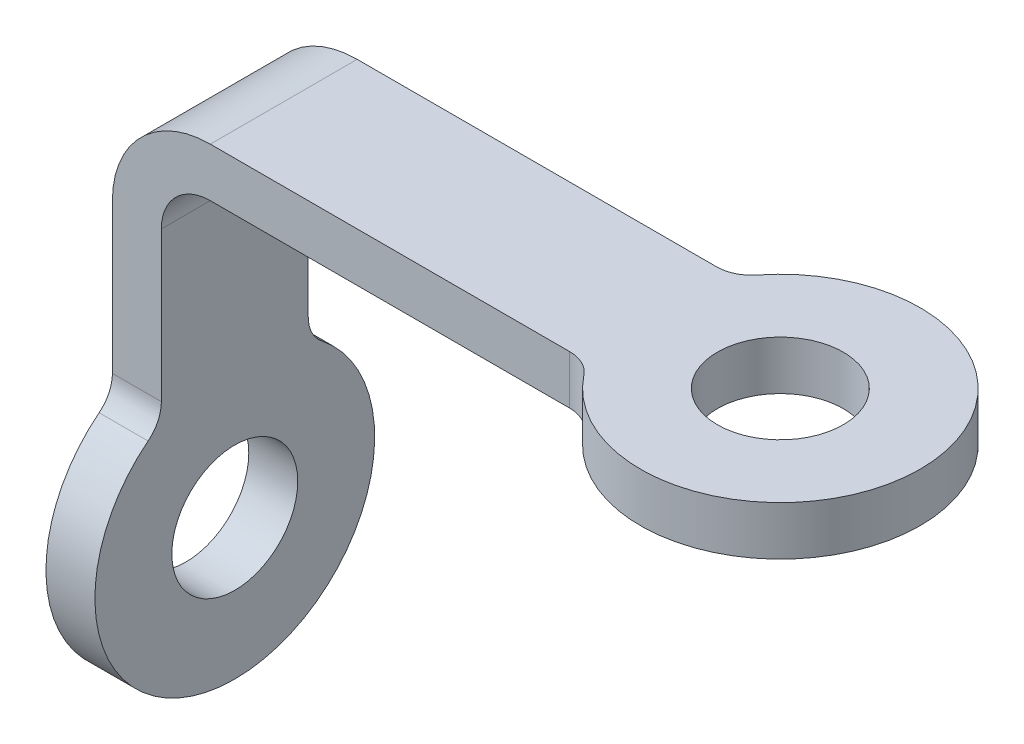
ISO-10303-21;
HEADER;
FILE_DESCRIPTION(('STEP AP214'),'2;1');
FILE_NAME('part.step','',(''),(''),'','','');
FILE_SCHEMA(('AUTOMOTIVE_DESIGN { 1 0 10303 214 1 1 1 1 }'));
ENDSEC;
DATA;
#1=APPLICATION_CONTEXT('core data for automotive mechanical design processes');
#2=APPLICATION_PROTOCOL_DEFINITION('international standard','automotive_design',2000,#1);
#3=PRODUCT_CONTEXT('',#1,'mechanical');
#4=PRODUCT('Part','Part','',(#3));
#5=PRODUCT_RELATED_PRODUCT_CATEGORY('part','',(#4));
#6=PRODUCT_DEFINITION_FORMATION('','',#4);
#7=PRODUCT_DEFINITION_CONTEXT('part definition',#1,'design');
#8=PRODUCT_DEFINITION('design','',#6,#7);
#9=PRODUCT_DEFINITION_SHAPE('','',#8);
#10=(LENGTH_UNIT() NAMED_UNIT(*) SI_UNIT(.MILLI.,.METRE.));
#11=(NAMED_UNIT(*) PLANE_ANGLE_UNIT() SI_UNIT($,.RADIAN.));
#12=(NAMED_UNIT(*) SI_UNIT($,.STERADIAN.) SOLID_ANGLE_UNIT());
#13=UNCERTAINTY_MEASURE_WITH_UNIT(LENGTH_MEASURE(1.E-05),#10,'distance_accuracy_value','');
#14=(GEOMETRIC_REPRESENTATION_CONTEXT(3) GLOBAL_UNCERTAINTY_ASSIGNED_CONTEXT((#13)) GLOBAL_UNIT_ASSIGNED_CONTEXT((#10,
#11,#12)) REPRESENTATION_CONTEXT('',''));
#15=CARTESIAN_POINT('',(0.,0.,0.));
#16=DIRECTION('',(0.,0.,1.));
#17=DIRECTION('',(1.,0.,0.));
#18=AXIS2_PLACEMENT_3D('',#15,#16,#17);
#19=CARTESIAN_POINT('',(0.,-7.,0.));
#20=DIRECTION('',(0.,1.,0.));
#21=DIRECTION('',(0.,0.,1.));
#22=AXIS2_PLACEMENT_3D('',#19,#20,#21);
#23=CYLINDRICAL_SURFACE('',#22,20.);
#24=CARTESIAN_POINT('',(0.,-7.,0.));
#25=DIRECTION('',(0.,1.,0.));
#26=DIRECTION('',(0.,0.,1.));
#27=AXIS2_PLACEMENT_3D('',#24,#25,#26);
#28=CIRCLE('',#27,20.);
#29=CARTESIAN_POINT('',(-15.6920361967464,-7.,12.4));
#30=VERTEX_POINT('',#29);
#31=CARTESIAN_POINT('',(-15.6920361967464,-7.,-12.4));
#32=VERTEX_POINT('',#31);
#33=EDGE_CURVE('E216',#30,#32,#28,.T.);
#34=ORIENTED_EDGE('',*,*,#33,.T.);
#35=DIRECTION('',(0.,1.,0.));
#36=VECTOR('',#35,1.);
#37=CARTESIAN_POINT('',(-15.6920361967464,-7.,-12.4));
#38=LINE('',#37,#36);
#39=CARTESIAN_POINT('',(-15.6920361967464,0.,-12.4));
#40=VERTEX_POINT('',#39);
#41=EDGE_CURVE('E149',#32,#40,#38,.T.);
#42=ORIENTED_EDGE('',*,*,#41,.T.);
#43=CARTESIAN_POINT('',(0.,0.,0.));
#44=DIRECTION('',(0.,1.,0.));
#45=DIRECTION('',(0.,0.,1.));
#46=AXIS2_PLACEMENT_3D('',#43,#44,#45);
#47=CIRCLE('',#46,20.);
#48=CARTESIAN_POINT('',(-15.6920361967464,0.,12.4));
#49=VERTEX_POINT('',#48);
#50=EDGE_CURVE('E135',#49,#40,#47,.T.);
#51=ORIENTED_EDGE('',*,*,#50,.F.);
#52=DIRECTION('',(0.,1.,0.));
#53=VECTOR('',#52,1.);
#54=CARTESIAN_POINT('',(-15.6920361967464,-7.,12.4));
#55=LINE('',#54,#53);
#56=EDGE_CURVE('E148',#49,#30,#55,.F.);
#57=ORIENTED_EDGE('',*,*,#56,.T.);
#58=EDGE_LOOP('',(#34,#42,#51,#57));
#59=FACE_BOUND('',#58,.T.);
#60=ADVANCED_FACE('F39',(#59),#23,.T.);
#61=CARTESIAN_POINT('',(-17.0220445305492,-7.,10.5));
#62=DIRECTION('',(0.,0.,1.));
#63=DIRECTION('',(1.,0.,0.));
#64=AXIS2_PLACEMENT_3D('',#61,#62,#63);
#65=PLANE('',#64);
#66=DIRECTION('',(1.,0.,0.));
#67=VECTOR('',#66,1.);
#68=CARTESIAN_POINT('',(-17.0220445305492,0.,10.5));
#69=LINE('',#68,#67);
#70=CARTESIAN_POINT('',(-71.,0.,10.5));
#71=VERTEX_POINT('',#70);
#72=CARTESIAN_POINT('',(-19.615045245933,0.,10.5));
#73=VERTEX_POINT('',#72);
#74=EDGE_CURVE('E134',#71,#73,#69,.T.);
#75=ORIENTED_EDGE('',*,*,#74,.F.);
#76=CARTESIAN_POINT('',(-71.,-14.,10.5));
#77=DIRECTION('',(0.,0.,1.));
#78=DIRECTION('',(1.,0.,0.));
#79=AXIS2_PLACEMENT_3D('',#76,#77,#78);
#80=CIRCLE('',#79,14.);
#81=CARTESIAN_POINT('',(-85.,-14.,10.5));
#82=VERTEX_POINT('',#81);
#83=EDGE_CURVE('E192',#71,#82,#80,.T.);
#84=ORIENTED_EDGE('',*,*,#83,.T.);
#85=DIRECTION('',(0.,1.,0.));
#86=VECTOR('',#85,1.);
#87=CARTESIAN_POINT('',(-85.,-7.,10.5));
#88=LINE('',#87,#86);
#89=CARTESIAN_POINT('',(-85.,-35.384954754067,10.5));
#90=VERTEX_POINT('',#89);
#91=EDGE_CURVE('E156',#90,#82,#88,.T.);
#92=ORIENTED_EDGE('',*,*,#91,.F.);
#93=DIRECTION('',(-1.,0.,0.));
#94=VECTOR('',#93,1.);
#95=CARTESIAN_POINT('',(-17.0220445305492,-35.384954754067,10.5));
#96=LINE('',#95,#94);
#97=CARTESIAN_POINT('',(-78.,-35.384954754067,10.4999999999999));
#98=VERTEX_POINT('',#97);
#99=EDGE_CURVE('E172',#90,#98,#96,.F.);
#100=ORIENTED_EDGE('',*,*,#99,.T.);
#101=DIRECTION('',(0.,-1.,0.));
#102=VECTOR('',#101,1.);
#103=CARTESIAN_POINT('',(-78.,0.,10.5));
#104=LINE('',#103,#102);
#105=CARTESIAN_POINT('',(-78.,-14.,10.5));
#106=VERTEX_POINT('',#105);
#107=EDGE_CURVE('E252',#106,#98,#104,.T.);
#108=ORIENTED_EDGE('',*,*,#107,.F.);
#109=CARTESIAN_POINT('',(-71.,-14.,10.5));
#110=DIRECTION('',(0.,0.,1.));
#111=DIRECTION('',(1.,0.,0.));
#112=AXIS2_PLACEMENT_3D('',#109,#110,#111);
#113=CIRCLE('',#112,7.);
#114=CARTESIAN_POINT('',(-71.,-7.,10.5));
#115=VERTEX_POINT('',#114);
#116=EDGE_CURVE('E11',#106,#115,#113,.F.);
#117=ORIENTED_EDGE('',*,*,#116,.T.);
#118=DIRECTION('',(1.,0.,0.));
#119=VECTOR('',#118,1.);
#120=CARTESIAN_POINT('',(-17.0220445305492,-7.,10.5));
#121=LINE('',#120,#119);
#122=CARTESIAN_POINT('',(-19.615045245933,-7.,10.5));
#123=VERTEX_POINT('',#122);
#124=EDGE_CURVE('E207',#115,#123,#121,.T.);
#125=ORIENTED_EDGE('',*,*,#124,.T.);
#126=DIRECTION('',(0.,-1.,0.));
#127=VECTOR('',#126,1.);
#128=CARTESIAN_POINT('',(-19.615045245933,0.,10.5));
#129=LINE('',#128,#127);
#130=EDGE_CURVE('E179',#123,#73,#129,.F.);
#131=ORIENTED_EDGE('',*,*,#130,.T.);
#132=EDGE_LOOP('',(#75,#84,#92,#100,#108,#117,#125,#131));
#133=FACE_BOUND('',#132,.T.);
#134=ADVANCED_FACE('F229',(#133),#65,.T.);
#135=CARTESIAN_POINT('',(-85.,-7.,-10.5));
#136=DIRECTION('',(-1.,0.,0.));
#137=DIRECTION('',(0.,0.,1.));
#138=AXIS2_PLACEMENT_3D('',#135,#136,#137);
#139=PLANE('',#138);
#140=ORIENTED_EDGE('',*,*,#91,.T.);
#141=DIRECTION('',(0.,0.,1.));
#142=VECTOR('',#141,1.);
#143=CARTESIAN_POINT('',(-85.,-14.,-10.5));
#144=LINE('',#143,#142);
#145=CARTESIAN_POINT('',(-85.,-14.,-10.5));
#146=VERTEX_POINT('',#145);
#147=EDGE_CURVE('E191',#82,#146,#144,.F.);
#148=ORIENTED_EDGE('',*,*,#147,.T.);
#149=DIRECTION('',(0.,1.,0.));
#150=VECTOR('',#149,1.);
#151=CARTESIAN_POINT('',(-85.,-7.,-10.5));
#152=LINE('',#151,#150);
#153=CARTESIAN_POINT('',(-85.,-35.3849547540669,-10.5));
#154=VERTEX_POINT('',#153);
#155=EDGE_CURVE('E161',#154,#146,#152,.T.);
#156=ORIENTED_EDGE('',*,*,#155,.F.);
#157=CARTESIAN_POINT('',(-85.,-35.3849547540669,-15.5));
#158=DIRECTION('',(-1.,0.,0.));
#159=DIRECTION('',(0.,0.,1.));
#160=AXIS2_PLACEMENT_3D('',#157,#158,#159);
#161=CIRCLE('',#160,5.);
#162=CARTESIAN_POINT('',(-85.,-39.3079638032535,-12.4));
#163=VERTEX_POINT('',#162);
#164=EDGE_CURVE('E181',#154,#163,#161,.F.);
#165=ORIENTED_EDGE('',*,*,#164,.T.);
#166=CARTESIAN_POINT('',(-85.,-55.,0.));
#167=DIRECTION('',(1.,0.,0.));
#168=DIRECTION('',(0.,0.,-1.));
#169=AXIS2_PLACEMENT_3D('',#166,#167,#168);
#170=CIRCLE('',#169,20.);
#171=CARTESIAN_POINT('',(-85.,-39.3079638032536,12.4));
#172=VERTEX_POINT('',#171);
#173=EDGE_CURVE('E236',#172,#163,#170,.T.);
#174=ORIENTED_EDGE('',*,*,#173,.F.);
#175=CARTESIAN_POINT('',(-85.,-35.384954754067,15.5));
#176=DIRECTION('',(-1.,0.,0.));
#177=DIRECTION('',(0.,0.,1.));
#178=AXIS2_PLACEMENT_3D('',#175,#176,#177);
#179=CIRCLE('',#178,5.);
#180=EDGE_CURVE('E190',#172,#90,#179,.F.);
#181=ORIENTED_EDGE('',*,*,#180,.T.);
#182=EDGE_LOOP('',(#140,#148,#156,#165,#174,#181));
#183=FACE_BOUND('',#182,.T.);
#184=CARTESIAN_POINT('',(-85.,-55.,0.));
#185=DIRECTION('',(1.,0.,0.));
#186=DIRECTION('',(0.,0.,-1.));
#187=AXIS2_PLACEMENT_3D('',#184,#185,#186);
#188=CIRCLE('',#187,9.);
#189=CARTESIAN_POINT('',(-85.,-55.,-9.00000000000006));
#190=VERTEX_POINT('',#189);
#191=EDGE_CURVE('E260',#190,#190,#188,.T.);
#192=ORIENTED_EDGE('',*,*,#191,.T.);
#193=EDGE_LOOP('',(#192));
#194=FACE_BOUND('',#193,.T.);
#195=ADVANCED_FACE('F232',(#183,#194),#139,.T.);
#196=CARTESIAN_POINT('',(-17.0220445305492,-7.,-10.5));
#197=DIRECTION('',(0.,0.,-1.));
#198=DIRECTION('',(-1.,0.,0.));
#199=AXIS2_PLACEMENT_3D('',#196,#197,#198);
#200=PLANE('',#199);
#201=ORIENTED_EDGE('',*,*,#155,.T.);
#202=CARTESIAN_POINT('',(-71.,-14.,-10.5));
#203=DIRECTION('',(0.,0.,-1.));
#204=DIRECTION('',(-1.,0.,0.));
#205=AXIS2_PLACEMENT_3D('',#202,#203,#204);
#206=CIRCLE('',#205,14.);
#207=CARTESIAN_POINT('',(-71.,0.,-10.5));
#208=VERTEX_POINT('',#207);
#209=EDGE_CURVE('E197',#146,#208,#206,.T.);
#210=ORIENTED_EDGE('',*,*,#209,.T.);
#211=DIRECTION('',(-1.,0.,0.));
#212=VECTOR('',#211,1.);
#213=CARTESIAN_POINT('',(-17.0220445305492,0.,-10.5));
#214=LINE('',#213,#212);
#215=CARTESIAN_POINT('',(-19.615045245933,0.,-10.5));
#216=VERTEX_POINT('',#215);
#217=EDGE_CURVE('E147',#216,#208,#214,.T.);
#218=ORIENTED_EDGE('',*,*,#217,.F.);
#219=DIRECTION('',(0.,-1.,0.));
#220=VECTOR('',#219,1.);
#221=CARTESIAN_POINT('',(-19.615045245933,-7.,-10.5));
#222=LINE('',#221,#220);
#223=CARTESIAN_POINT('',(-19.615045245933,-7.,-10.5));
#224=VERTEX_POINT('',#223);
#225=EDGE_CURVE('E170',#216,#224,#222,.T.);
#226=ORIENTED_EDGE('',*,*,#225,.T.);
#227=DIRECTION('',(-1.,0.,0.));
#228=VECTOR('',#227,1.);
#229=CARTESIAN_POINT('',(-17.0220445305492,-7.,-10.5));
#230=LINE('',#229,#228);
#231=CARTESIAN_POINT('',(-71.,-7.,-10.5));
#232=VERTEX_POINT('',#231);
#233=EDGE_CURVE('E210',#224,#232,#230,.T.);
#234=ORIENTED_EDGE('',*,*,#233,.T.);
#235=CARTESIAN_POINT('',(-71.,-14.,-10.5));
#236=DIRECTION('',(0.,0.,-1.));
#237=DIRECTION('',(-1.,0.,0.));
#238=AXIS2_PLACEMENT_3D('',#235,#236,#237);
#239=CIRCLE('',#238,7.);
#240=CARTESIAN_POINT('',(-78.,-14.,-10.5000000000001));
#241=VERTEX_POINT('',#240);
#242=EDGE_CURVE('E50',#232,#241,#239,.F.);
#243=ORIENTED_EDGE('',*,*,#242,.T.);
#244=DIRECTION('',(0.,1.,0.));
#245=VECTOR('',#244,1.);
#246=CARTESIAN_POINT('',(-78.,-37.9779554694508,-10.5000000000001));
#247=LINE('',#246,#245);
#248=CARTESIAN_POINT('',(-78.,-35.3849547540669,-10.5000000000001));
#249=VERTEX_POINT('',#248);
#250=EDGE_CURVE('E246',#249,#241,#247,.T.);
#251=ORIENTED_EDGE('',*,*,#250,.F.);
#252=DIRECTION('',(-1.,0.,0.));
#253=VECTOR('',#252,1.);
#254=CARTESIAN_POINT('',(-17.0220445305492,-35.3849547540669,-10.5));
#255=LINE('',#254,#253);
#256=EDGE_CURVE('E158',#249,#154,#255,.T.);
#257=ORIENTED_EDGE('',*,*,#256,.T.);
#258=EDGE_LOOP('',(#201,#210,#218,#226,#234,#243,#251,#257));
#259=FACE_BOUND('',#258,.T.);
#260=ADVANCED_FACE('F213',(#259),#200,.T.);
#261=CARTESIAN_POINT('',(0.,-7.,0.));
#262=DIRECTION('',(0.,1.,0.));
#263=DIRECTION('',(0.,0.,1.));
#264=AXIS2_PLACEMENT_3D('',#261,#262,#263);
#265=PLANE('',#264);
#266=CARTESIAN_POINT('',(0.,-7.,0.));
#267=DIRECTION('',(0.,1.,0.));
#268=DIRECTION('',(0.,0.,1.));
#269=AXIS2_PLACEMENT_3D('',#266,#267,#268);
#270=CIRCLE('',#269,9.);
#271=CARTESIAN_POINT('',(0.,-7.,9.));
#272=VERTEX_POINT('',#271);
#273=EDGE_CURVE('E151',#272,#272,#270,.T.);
#274=ORIENTED_EDGE('',*,*,#273,.T.);
#275=EDGE_LOOP('',(#274));
#276=FACE_BOUND('',#275,.T.);
#277=ORIENTED_EDGE('',*,*,#124,.F.);
#278=DIRECTION('',(0.,0.,-1.));
#279=VECTOR('',#278,1.);
#280=CARTESIAN_POINT('',(-71.,-7.,0.));
#281=LINE('',#280,#279);
#282=EDGE_CURVE('E200',#115,#232,#281,.T.);
#283=ORIENTED_EDGE('',*,*,#282,.T.);
#284=ORIENTED_EDGE('',*,*,#233,.F.);
#285=CARTESIAN_POINT('',(-19.615045245933,-7.,-15.5));
#286=DIRECTION('',(0.,1.,0.));
#287=DIRECTION('',(0.,0.,1.));
#288=AXIS2_PLACEMENT_3D('',#285,#286,#287);
#289=CIRCLE('',#288,5.);
#290=EDGE_CURVE('E182',#224,#32,#289,.T.);
#291=ORIENTED_EDGE('',*,*,#290,.T.);
#292=ORIENTED_EDGE('',*,*,#33,.F.);
#293=CARTESIAN_POINT('',(-19.615045245933,-7.,15.5));
#294=DIRECTION('',(0.,1.,0.));
#295=DIRECTION('',(0.,0.,1.));
#296=AXIS2_PLACEMENT_3D('',#293,#294,#295);
#297=CIRCLE('',#296,5.);
#298=EDGE_CURVE('E136',#30,#123,#297,.T.);
#299=ORIENTED_EDGE('',*,*,#298,.T.);
#300=EDGE_LOOP('',(#277,#283,#284,#291,#292,#299));
#301=FACE_BOUND('',#300,.T.);
#302=ADVANCED_FACE('F206',(#276,#301),#265,.F.);
#303=CARTESIAN_POINT('',(0.,0.,0.));
#304=DIRECTION('',(0.,1.,0.));
#305=DIRECTION('',(0.,0.,1.));
#306=AXIS2_PLACEMENT_3D('',#303,#304,#305);
#307=PLANE('',#306);
#308=ORIENTED_EDGE('',*,*,#217,.T.);
#309=DIRECTION('',(0.,0.,1.));
#310=VECTOR('',#309,1.);
#311=CARTESIAN_POINT('',(-71.,0.,0.));
#312=LINE('',#311,#310);
#313=EDGE_CURVE('E193',#208,#71,#312,.T.);
#314=ORIENTED_EDGE('',*,*,#313,.T.);
#315=ORIENTED_EDGE('',*,*,#74,.T.);
#316=CARTESIAN_POINT('',(-19.615045245933,0.,15.5));
#317=DIRECTION('',(0.,1.,0.));
#318=DIRECTION('',(0.,0.,1.));
#319=AXIS2_PLACEMENT_3D('',#316,#317,#318);
#320=CIRCLE('',#319,5.);
#321=EDGE_CURVE('E130',#73,#49,#320,.F.);
#322=ORIENTED_EDGE('',*,*,#321,.T.);
#323=ORIENTED_EDGE('',*,*,#50,.T.);
#324=CARTESIAN_POINT('',(-19.615045245933,0.,-15.5));
#325=DIRECTION('',(0.,1.,0.));
#326=DIRECTION('',(0.,0.,1.));
#327=AXIS2_PLACEMENT_3D('',#324,#325,#326);
#328=CIRCLE('',#327,5.);
#329=EDGE_CURVE('E180',#40,#216,#328,.F.);
#330=ORIENTED_EDGE('',*,*,#329,.T.);
#331=EDGE_LOOP('',(#308,#314,#315,#322,#323,#330));
#332=FACE_BOUND('',#331,.T.);
#333=CARTESIAN_POINT('',(0.,0.,0.));
#334=DIRECTION('',(0.,1.,0.));
#335=DIRECTION('',(0.,0.,1.));
#336=AXIS2_PLACEMENT_3D('',#333,#334,#335);
#337=CIRCLE('',#336,9.);
#338=CARTESIAN_POINT('',(0.,0.,9.));
#339=VERTEX_POINT('',#338);
#340=EDGE_CURVE('E257',#339,#339,#337,.T.);
#341=ORIENTED_EDGE('',*,*,#340,.F.);
#342=EDGE_LOOP('',(#341));
#343=FACE_BOUND('',#342,.T.);
#344=ADVANCED_FACE('F128',(#332,#343),#307,.T.);
#345=CARTESIAN_POINT('',(0.,-7.,0.));
#346=DIRECTION('',(0.,1.,0.));
#347=DIRECTION('',(0.,0.,1.));
#348=AXIS2_PLACEMENT_3D('',#345,#346,#347);
#349=CYLINDRICAL_SURFACE('',#348,9.);
#350=ORIENTED_EDGE('',*,*,#273,.F.);
#351=EDGE_LOOP('',(#350));
#352=FACE_BOUND('',#351,.T.);
#353=ORIENTED_EDGE('',*,*,#340,.T.);
#354=EDGE_LOOP('',(#353));
#355=FACE_BOUND('',#354,.T.);
#356=ADVANCED_FACE('F266',(#352,#355),#349,.F.);
#357=CARTESIAN_POINT('',(-78.,-55.,0.));
#358=DIRECTION('',(1.,0.,0.));
#359=DIRECTION('',(0.,0.,-1.));
#360=AXIS2_PLACEMENT_3D('',#357,#358,#359);
#361=PLANE('',#360);
#362=CARTESIAN_POINT('',(-78.,-55.,0.));
#363=DIRECTION('',(1.,0.,0.));
#364=DIRECTION('',(0.,0.,-1.));
#365=AXIS2_PLACEMENT_3D('',#362,#363,#364);
#366=CIRCLE('',#365,9.);
#367=CARTESIAN_POINT('',(-78.,-55.,-9.00000000000006));
#368=VERTEX_POINT('',#367);
#369=EDGE_CURVE('E255',#368,#368,#366,.T.);
#370=ORIENTED_EDGE('',*,*,#369,.F.);
#371=EDGE_LOOP('',(#370));
#372=FACE_BOUND('',#371,.T.);
#373=ORIENTED_EDGE('',*,*,#250,.T.);
#374=DIRECTION('',(0.,0.,-1.));
#375=VECTOR('',#374,1.);
#376=CARTESIAN_POINT('',(-78.,-14.,0.));
#377=LINE('',#376,#375);
#378=EDGE_CURVE('E58',#241,#106,#377,.F.);
#379=ORIENTED_EDGE('',*,*,#378,.T.);
#380=ORIENTED_EDGE('',*,*,#107,.T.);
#381=CARTESIAN_POINT('',(-78.,-35.384954754067,15.5));
#382=DIRECTION('',(1.,0.,0.));
#383=DIRECTION('',(0.,0.,-1.));
#384=AXIS2_PLACEMENT_3D('',#381,#382,#383);
#385=CIRCLE('',#384,5.);
#386=CARTESIAN_POINT('',(-78.,-39.3079638032536,12.4));
#387=VERTEX_POINT('',#386);
#388=EDGE_CURVE('E187',#98,#387,#385,.F.);
#389=ORIENTED_EDGE('',*,*,#388,.T.);
#390=CARTESIAN_POINT('',(-78.,-55.,0.));
#391=DIRECTION('',(1.,0.,0.));
#392=DIRECTION('',(0.,0.,-1.));
#393=AXIS2_PLACEMENT_3D('',#390,#391,#392);
#394=CIRCLE('',#393,20.);
#395=CARTESIAN_POINT('',(-78.,-39.3079638032535,-12.4));
#396=VERTEX_POINT('',#395);
#397=EDGE_CURVE('E247',#387,#396,#394,.T.);
#398=ORIENTED_EDGE('',*,*,#397,.T.);
#399=CARTESIAN_POINT('',(-78.,-35.3849547540669,-15.5));
#400=DIRECTION('',(1.,0.,0.));
#401=DIRECTION('',(0.,0.,-1.));
#402=AXIS2_PLACEMENT_3D('',#399,#400,#401);
#403=CIRCLE('',#402,5.);
#404=EDGE_CURVE('E143',#396,#249,#403,.F.);
#405=ORIENTED_EDGE('',*,*,#404,.T.);
#406=EDGE_LOOP('',(#373,#379,#380,#389,#398,#405));
#407=FACE_BOUND('',#406,.T.);
#408=ADVANCED_FACE('F273',(#372,#407),#361,.T.);
#409=CARTESIAN_POINT('',(-78.,-55.,0.));
#410=DIRECTION('',(-1.,0.,0.));
#411=DIRECTION('',(0.,0.,1.));
#412=AXIS2_PLACEMENT_3D('',#409,#410,#411);
#413=CYLINDRICAL_SURFACE('',#412,20.);
#414=ORIENTED_EDGE('',*,*,#173,.T.);
#415=DIRECTION('',(-1.,0.,0.));
#416=VECTOR('',#415,1.);
#417=CARTESIAN_POINT('',(-78.,-39.3079638032535,-12.4));
#418=LINE('',#417,#416);
#419=EDGE_CURVE('E175',#163,#396,#418,.F.);
#420=ORIENTED_EDGE('',*,*,#419,.T.);
#421=ORIENTED_EDGE('',*,*,#397,.F.);
#422=DIRECTION('',(-1.,0.,0.));
#423=VECTOR('',#422,1.);
#424=CARTESIAN_POINT('',(-78.,-39.3079638032536,12.4));
#425=LINE('',#424,#423);
#426=EDGE_CURVE('E166',#387,#172,#425,.T.);
#427=ORIENTED_EDGE('',*,*,#426,.T.);
#428=EDGE_LOOP('',(#414,#420,#421,#427));
#429=FACE_BOUND('',#428,.T.);
#430=ADVANCED_FACE('F244',(#429),#413,.T.);
#431=CARTESIAN_POINT('',(-78.,-55.,0.));
#432=DIRECTION('',(-1.,0.,0.));
#433=DIRECTION('',(0.,0.,1.));
#434=AXIS2_PLACEMENT_3D('',#431,#432,#433);
#435=CYLINDRICAL_SURFACE('',#434,9.);
#436=ORIENTED_EDGE('',*,*,#369,.T.);
#437=EDGE_LOOP('',(#436));
#438=FACE_BOUND('',#437,.T.);
#439=ORIENTED_EDGE('',*,*,#191,.F.);
#440=EDGE_LOOP('',(#439));
#441=FACE_BOUND('',#440,.T.);
#442=ADVANCED_FACE('F293',(#438,#441),#435,.F.);
#443=CARTESIAN_POINT('',(-19.615045245933,-7.,-15.5));
#444=DIRECTION('',(0.,1.,0.));
#445=DIRECTION('',(0.,0.,1.));
#446=AXIS2_PLACEMENT_3D('',#443,#444,#445);
#447=CYLINDRICAL_SURFACE('',#446,5.);
#448=ORIENTED_EDGE('',*,*,#290,.F.);
#449=ORIENTED_EDGE('',*,*,#225,.F.);
#450=ORIENTED_EDGE('',*,*,#329,.F.);
#451=ORIENTED_EDGE('',*,*,#41,.F.);
#452=EDGE_LOOP('',(#448,#449,#450,#451));
#453=FACE_BOUND('',#452,.T.);
#454=ADVANCED_FACE('F292',(#453),#447,.F.);
#455=CARTESIAN_POINT('',(-78.,-35.3849547540669,-15.5));
#456=DIRECTION('',(-1.,0.,0.));
#457=DIRECTION('',(0.,0.,1.));
#458=AXIS2_PLACEMENT_3D('',#455,#456,#457);
#459=CYLINDRICAL_SURFACE('',#458,5.);
#460=ORIENTED_EDGE('',*,*,#404,.F.);
#461=ORIENTED_EDGE('',*,*,#419,.F.);
#462=ORIENTED_EDGE('',*,*,#164,.F.);
#463=ORIENTED_EDGE('',*,*,#256,.F.);
#464=EDGE_LOOP('',(#460,#461,#462,#463));
#465=FACE_BOUND('',#464,.T.);
#466=ADVANCED_FACE('F294',(#465),#459,.F.);
#467=CARTESIAN_POINT('',(-19.615045245933,-7.,15.5));
#468=DIRECTION('',(0.,1.,0.));
#469=DIRECTION('',(0.,0.,1.));
#470=AXIS2_PLACEMENT_3D('',#467,#468,#469);
#471=CYLINDRICAL_SURFACE('',#470,5.);
#472=ORIENTED_EDGE('',*,*,#298,.F.);
#473=ORIENTED_EDGE('',*,*,#56,.F.);
#474=ORIENTED_EDGE('',*,*,#321,.F.);
#475=ORIENTED_EDGE('',*,*,#130,.F.);
#476=EDGE_LOOP('',(#472,#473,#474,#475));
#477=FACE_BOUND('',#476,.T.);
#478=ADVANCED_FACE('F152',(#477),#471,.F.);
#479=CARTESIAN_POINT('',(-78.,-35.384954754067,15.5));
#480=DIRECTION('',(-1.,0.,0.));
#481=DIRECTION('',(0.,0.,1.));
#482=AXIS2_PLACEMENT_3D('',#479,#480,#481);
#483=CYLINDRICAL_SURFACE('',#482,5.);
#484=ORIENTED_EDGE('',*,*,#388,.F.);
#485=ORIENTED_EDGE('',*,*,#99,.F.);
#486=ORIENTED_EDGE('',*,*,#180,.F.);
#487=ORIENTED_EDGE('',*,*,#426,.F.);
#488=EDGE_LOOP('',(#484,#485,#486,#487));
#489=FACE_BOUND('',#488,.T.);
#490=ADVANCED_FACE('F245',(#489),#483,.F.);
#491=CARTESIAN_POINT('',(-71.,-14.,0.));
#492=DIRECTION('',(0.,0.,1.));
#493=DIRECTION('',(1.,0.,0.));
#494=AXIS2_PLACEMENT_3D('',#491,#492,#493);
#495=CYLINDRICAL_SURFACE('',#494,14.);
#496=ORIENTED_EDGE('',*,*,#209,.F.);
#497=ORIENTED_EDGE('',*,*,#147,.F.);
#498=ORIENTED_EDGE('',*,*,#83,.F.);
#499=ORIENTED_EDGE('',*,*,#313,.F.);
#500=EDGE_LOOP('',(#496,#497,#498,#499));
#501=FACE_BOUND('',#500,.T.);
#502=ADVANCED_FACE('F228',(#501),#495,.T.);
#503=CARTESIAN_POINT('',(-71.,-14.,0.));
#504=DIRECTION('',(0.,0.,-1.));
#505=DIRECTION('',(-1.,0.,0.));
#506=AXIS2_PLACEMENT_3D('',#503,#504,#505);
#507=CYLINDRICAL_SURFACE('',#506,7.);
#508=ORIENTED_EDGE('',*,*,#116,.F.);
#509=ORIENTED_EDGE('',*,*,#378,.F.);
#510=ORIENTED_EDGE('',*,*,#242,.F.);
#511=ORIENTED_EDGE('',*,*,#282,.F.);
#512=EDGE_LOOP('',(#508,#509,#510,#511));
#513=FACE_BOUND('',#512,.T.);
#514=ADVANCED_FACE('F41',(#513),#507,.F.);
#515=CLOSED_SHELL('',(#60,#134,#195,#260,#302,#344,#356,#408,#430,#442,#454,#466,#478,#490,#502,#514));
#516=MANIFOLD_SOLID_BREP('B2',#515);
#517=ADVANCED_BREP_SHAPE_REPRESENTATION('',(#18,#516),#14);
#518=SHAPE_DEFINITION_REPRESENTATION(#9,#517);
ENDSEC;
END-ISO-10303-21;
